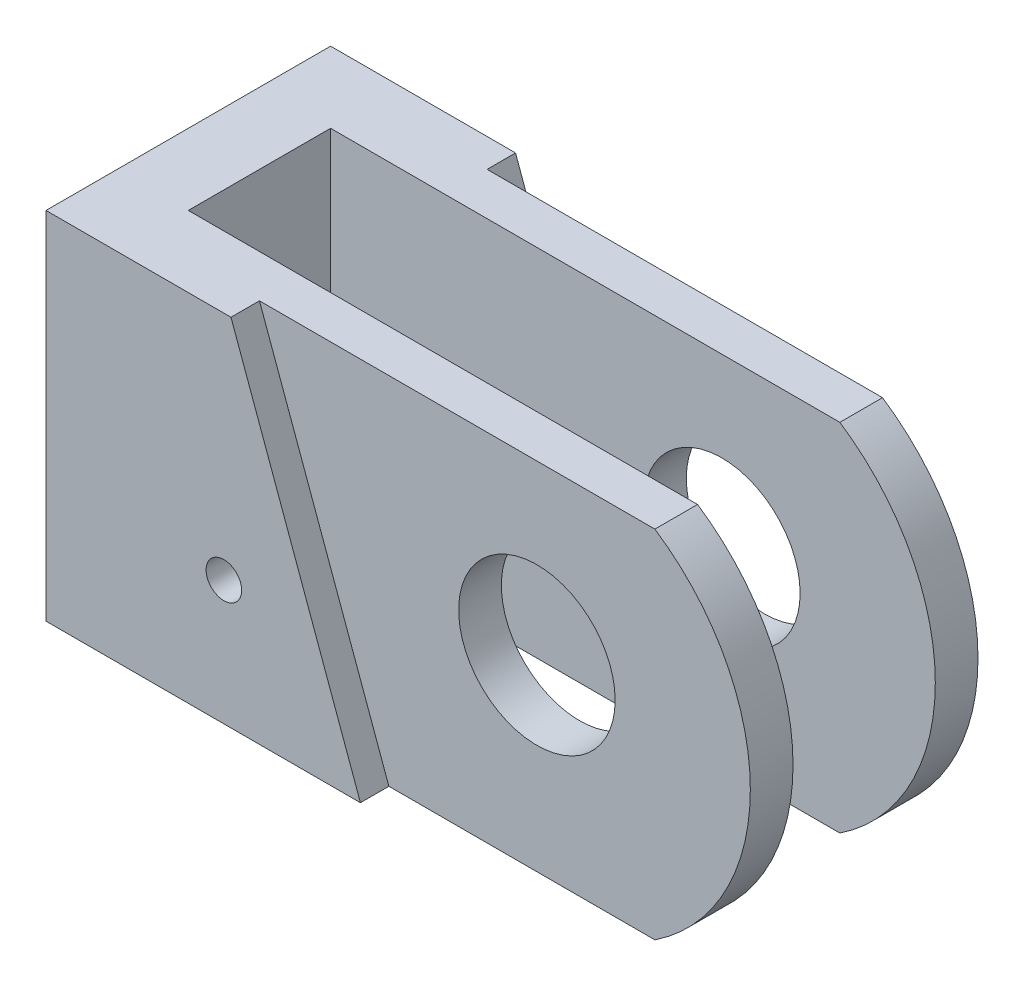
ISO-10303-21;
HEADER;
FILE_DESCRIPTION(('STEP AP214'),'2;1');
FILE_NAME('part.step','',(''),(''),'','','');
FILE_SCHEMA(('AUTOMOTIVE_DESIGN { 1 0 10303 214 1 1 1 1 }'));
ENDSEC;
DATA;
#1=APPLICATION_CONTEXT('core data for automotive mechanical design processes');
#2=APPLICATION_PROTOCOL_DEFINITION('international standard','automotive_design',2000,#1);
#3=PRODUCT_CONTEXT('',#1,'mechanical');
#4=PRODUCT('Part','Part','',(#3));
#5=PRODUCT_RELATED_PRODUCT_CATEGORY('part','',(#4));
#6=PRODUCT_DEFINITION_FORMATION('','',#4);
#7=PRODUCT_DEFINITION_CONTEXT('part definition',#1,'design');
#8=PRODUCT_DEFINITION('design','',#6,#7);
#9=PRODUCT_DEFINITION_SHAPE('','',#8);
#10=(LENGTH_UNIT() NAMED_UNIT(*) SI_UNIT(.MILLI.,.METRE.));
#11=(NAMED_UNIT(*) PLANE_ANGLE_UNIT() SI_UNIT($,.RADIAN.));
#12=(NAMED_UNIT(*) SI_UNIT($,.STERADIAN.) SOLID_ANGLE_UNIT());
#13=UNCERTAINTY_MEASURE_WITH_UNIT(LENGTH_MEASURE(1.E-05),#10,'distance_accuracy_value','');
#14=(GEOMETRIC_REPRESENTATION_CONTEXT(3) GLOBAL_UNCERTAINTY_ASSIGNED_CONTEXT((#13)) GLOBAL_UNIT_ASSIGNED_CONTEXT((#10,
#11,#12)) REPRESENTATION_CONTEXT('',''));
#15=CARTESIAN_POINT('',(0.,0.,0.));
#16=DIRECTION('',(0.,0.,1.));
#17=DIRECTION('',(1.,0.,0.));
#18=AXIS2_PLACEMENT_3D('',#15,#16,#17);
#19=CARTESIAN_POINT('',(10.,0.,0.));
#20=DIRECTION('',(1.,0.,0.));
#21=DIRECTION('',(0.,1.,0.));
#22=AXIS2_PLACEMENT_3D('',#19,#20,#21);
#23=PLANE('',#22);
#24=CARTESIAN_POINT('',(10.,-25.,20.));
#25=DIRECTION('',(1.,0.,0.));
#26=DIRECTION('',(0.,1.,0.));
#27=AXIS2_PLACEMENT_3D('',#24,#25,#26);
#28=CIRCLE('',#27,10.);
#29=CARTESIAN_POINT('',(10.,-25.,30.));
#30=VERTEX_POINT('',#29);
#31=CARTESIAN_POINT('',(10.,-25.,10.));
#32=VERTEX_POINT('',#31);
#33=EDGE_CURVE('E64',#30,#32,#28,.T.);
#34=ORIENTED_EDGE('',*,*,#33,.F.);
#35=DIRECTION('',(0.,-1.,0.));
#36=VECTOR('',#35,1.);
#37=CARTESIAN_POINT('',(10.,-50.,30.));
#38=LINE('',#37,#36);
#39=CARTESIAN_POINT('',(10.,-50.,30.));
#40=VERTEX_POINT('',#39);
#41=EDGE_CURVE('E151',#30,#40,#38,.T.);
#42=ORIENTED_EDGE('',*,*,#41,.T.);
#43=DIRECTION('',(0.,0.,1.));
#44=VECTOR('',#43,1.);
#45=CARTESIAN_POINT('',(10.,-50.,40.));
#46=LINE('',#45,#44);
#47=CARTESIAN_POINT('',(10.,-50.,10.));
#48=VERTEX_POINT('',#47);
#49=EDGE_CURVE('E188',#48,#40,#46,.T.);
#50=ORIENTED_EDGE('',*,*,#49,.F.);
#51=DIRECTION('',(0.,-1.,0.));
#52=VECTOR('',#51,1.);
#53=CARTESIAN_POINT('',(10.,-50.,10.));
#54=LINE('',#53,#52);
#55=EDGE_CURVE('E153',#32,#48,#54,.T.);
#56=ORIENTED_EDGE('',*,*,#55,.F.);
#57=EDGE_LOOP('',(#34,#42,#50,#56));
#58=FACE_BOUND('',#57,.T.);
#59=ADVANCED_FACE('F44',(#58),#23,.T.);
#60=CARTESIAN_POINT('',(65.,-25.,10.));
#61=DIRECTION('',(0.,0.,-1.));
#62=DIRECTION('',(-1.,0.,0.));
#63=AXIS2_PLACEMENT_3D('',#60,#61,#62);
#64=CYLINDRICAL_SURFACE('',#63,30.);
#65=CARTESIAN_POINT('',(65.,-25.,4.));
#66=DIRECTION('',(0.,0.,-1.));
#67=DIRECTION('',(-1.,0.,0.));
#68=AXIS2_PLACEMENT_3D('',#65,#66,#67);
#69=CIRCLE('',#68,30.);
#70=CARTESIAN_POINT('',(81.583123951777,0.,4.));
#71=VERTEX_POINT('',#70);
#72=CARTESIAN_POINT('',(81.583123951777,-50.,4.));
#73=VERTEX_POINT('',#72);
#74=EDGE_CURVE('E252',#71,#73,#69,.T.);
#75=ORIENTED_EDGE('',*,*,#74,.F.);
#76=DIRECTION('',(0.,0.,-1.));
#77=VECTOR('',#76,1.);
#78=CARTESIAN_POINT('',(81.583123951777,0.,10.));
#79=LINE('',#78,#77);
#80=CARTESIAN_POINT('',(81.583123951777,0.,10.));
#81=VERTEX_POINT('',#80);
#82=EDGE_CURVE('E209',#81,#71,#79,.T.);
#83=ORIENTED_EDGE('',*,*,#82,.F.);
#84=CARTESIAN_POINT('',(65.,-25.,10.));
#85=DIRECTION('',(0.,0.,1.));
#86=DIRECTION('',(1.,0.,0.));
#87=AXIS2_PLACEMENT_3D('',#84,#85,#86);
#88=CIRCLE('',#87,30.);
#89=CARTESIAN_POINT('',(81.583123951777,-50.,10.));
#90=VERTEX_POINT('',#89);
#91=EDGE_CURVE('E207',#90,#81,#88,.T.);
#92=ORIENTED_EDGE('',*,*,#91,.F.);
#93=DIRECTION('',(0.,0.,-1.));
#94=VECTOR('',#93,1.);
#95=CARTESIAN_POINT('',(81.583123951777,-50.,10.));
#96=LINE('',#95,#94);
#97=EDGE_CURVE('E218',#90,#73,#96,.T.);
#98=ORIENTED_EDGE('',*,*,#97,.T.);
#99=EDGE_LOOP('',(#75,#83,#92,#98));
#100=FACE_BOUND('',#99,.T.);
#101=ADVANCED_FACE('F297',(#100),#64,.T.);
#102=CARTESIAN_POINT('',(65.,-25.,30.));
#103=DIRECTION('',(0.,0.,1.));
#104=DIRECTION('',(1.,0.,0.));
#105=AXIS2_PLACEMENT_3D('',#102,#103,#104);
#106=CYLINDRICAL_SURFACE('',#105,30.);
#107=DIRECTION('',(0.,0.,1.));
#108=VECTOR('',#107,1.);
#109=CARTESIAN_POINT('',(81.583123951777,0.,30.));
#110=LINE('',#109,#108);
#111=CARTESIAN_POINT('',(81.583123951777,0.,30.));
#112=VERTEX_POINT('',#111);
#113=CARTESIAN_POINT('',(81.583123951777,0.,36.));
#114=VERTEX_POINT('',#113);
#115=EDGE_CURVE('E185',#112,#114,#110,.T.);
#116=ORIENTED_EDGE('',*,*,#115,.T.);
#117=CARTESIAN_POINT('',(65.,-25.,36.));
#118=DIRECTION('',(0.,0.,1.));
#119=DIRECTION('',(1.,0.,0.));
#120=AXIS2_PLACEMENT_3D('',#117,#118,#119);
#121=CIRCLE('',#120,30.);
#122=CARTESIAN_POINT('',(81.583123951777,-50.,36.));
#123=VERTEX_POINT('',#122);
#124=EDGE_CURVE('E269',#123,#114,#121,.T.);
#125=ORIENTED_EDGE('',*,*,#124,.F.);
#126=DIRECTION('',(0.,0.,1.));
#127=VECTOR('',#126,1.);
#128=CARTESIAN_POINT('',(81.583123951777,-50.,30.));
#129=LINE('',#128,#127);
#130=CARTESIAN_POINT('',(81.583123951777,-50.,30.));
#131=VERTEX_POINT('',#130);
#132=EDGE_CURVE('E181',#131,#123,#129,.T.);
#133=ORIENTED_EDGE('',*,*,#132,.F.);
#134=CARTESIAN_POINT('',(65.,-25.,30.));
#135=DIRECTION('',(0.,0.,1.));
#136=DIRECTION('',(1.,0.,0.));
#137=AXIS2_PLACEMENT_3D('',#134,#135,#136);
#138=CIRCLE('',#137,30.);
#139=EDGE_CURVE('E171',#131,#112,#138,.T.);
#140=ORIENTED_EDGE('',*,*,#139,.T.);
#141=EDGE_LOOP('',(#116,#125,#133,#140));
#142=FACE_BOUND('',#141,.T.);
#143=ADVANCED_FACE('F307',(#142),#106,.T.);
#144=EDGE_CURVE('E136',#32,#30,#28,.T.);
#145=ORIENTED_EDGE('',*,*,#144,.F.);
#146=CARTESIAN_POINT('',(10.,0.,10.));
#147=VERTEX_POINT('',#146);
#148=EDGE_CURVE('E189',#147,#32,#54,.T.);
#149=ORIENTED_EDGE('',*,*,#148,.F.);
#150=DIRECTION('',(0.,0.,-1.));
#151=VECTOR('',#150,1.);
#152=CARTESIAN_POINT('',(10.,0.,10.));
#153=LINE('',#152,#151);
#154=CARTESIAN_POINT('',(10.,0.,30.));
#155=VERTEX_POINT('',#154);
#156=EDGE_CURVE('E167',#155,#147,#153,.T.);
#157=ORIENTED_EDGE('',*,*,#156,.F.);
#158=EDGE_CURVE('E158',#155,#30,#38,.T.);
#159=ORIENTED_EDGE('',*,*,#158,.T.);
#160=EDGE_LOOP('',(#145,#149,#157,#159));
#161=FACE_BOUND('',#160,.T.);
#162=ADVANCED_FACE('F169',(#161),#23,.T.);
#163=CARTESIAN_POINT('',(65.,-25.,10.));
#164=DIRECTION('',(0.,0.,1.));
#165=DIRECTION('',(1.,0.,0.));
#166=AXIS2_PLACEMENT_3D('',#163,#164,#165);
#167=PLANE('',#166);
#168=CARTESIAN_POINT('',(25.,-32.5,10.));
#169=DIRECTION('',(0.,0.,1.));
#170=DIRECTION('',(1.,0.,0.));
#171=AXIS2_PLACEMENT_3D('',#168,#169,#170);
#172=CIRCLE('',#171,2.5);
#173=CARTESIAN_POINT('',(27.5,-32.5,10.));
#174=VERTEX_POINT('',#173);
#175=EDGE_CURVE('E354',#174,#174,#172,.T.);
#176=ORIENTED_EDGE('',*,*,#175,.F.);
#177=EDGE_LOOP('',(#176));
#178=FACE_BOUND('',#177,.T.);
#179=ORIENTED_EDGE('',*,*,#148,.T.);
#180=ORIENTED_EDGE('',*,*,#55,.T.);
#181=DIRECTION('',(1.,0.,0.));
#182=VECTOR('',#181,1.);
#183=CARTESIAN_POINT('',(0.,-50.,10.));
#184=LINE('',#183,#182);
#185=EDGE_CURVE('E205',#48,#90,#184,.T.);
#186=ORIENTED_EDGE('',*,*,#185,.T.);
#187=ORIENTED_EDGE('',*,*,#91,.T.);
#188=DIRECTION('',(-1.,0.,0.));
#189=VECTOR('',#188,1.);
#190=CARTESIAN_POINT('',(0.,0.,10.));
#191=LINE('',#190,#189);
#192=EDGE_CURVE('E199',#81,#147,#191,.T.);
#193=ORIENTED_EDGE('',*,*,#192,.T.);
#194=EDGE_LOOP('',(#179,#180,#186,#187,#193));
#195=FACE_BOUND('',#194,.T.);
#196=CARTESIAN_POINT('',(65.,-23.6191908710067,10.));
#197=DIRECTION('',(0.,0.,1.));
#198=DIRECTION('',(1.,0.,0.));
#199=AXIS2_PLACEMENT_3D('',#196,#197,#198);
#200=CIRCLE('',#199,11.);
#201=CARTESIAN_POINT('',(76.,-23.6191908710067,10.));
#202=VERTEX_POINT('',#201);
#203=EDGE_CURVE('E230',#202,#202,#200,.T.);
#204=ORIENTED_EDGE('',*,*,#203,.F.);
#205=EDGE_LOOP('',(#204));
#206=FACE_BOUND('',#205,.T.);
#207=ADVANCED_FACE('F304',(#178,#195,#206),#167,.T.);
#208=CARTESIAN_POINT('',(0.,0.,10.));
#209=DIRECTION('',(1.,0.,0.));
#210=DIRECTION('',(0.,1.,0.));
#211=AXIS2_PLACEMENT_3D('',#208,#209,#210);
#212=PLANE('',#211);
#213=CARTESIAN_POINT('',(0.,-25.,20.));
#214=DIRECTION('',(-1.,0.,0.));
#215=DIRECTION('',(0.,-1.,0.));
#216=AXIS2_PLACEMENT_3D('',#213,#214,#215);
#217=CIRCLE('',#216,15.);
#218=CARTESIAN_POINT('',(0.,-40.,20.));
#219=VERTEX_POINT('',#218);
#220=EDGE_CURVE('E154',#219,#219,#217,.T.);
#221=ORIENTED_EDGE('',*,*,#220,.F.);
#222=EDGE_LOOP('',(#221));
#223=FACE_BOUND('',#222,.T.);
#224=DIRECTION('',(0.,-1.,0.));
#225=VECTOR('',#224,1.);
#226=CARTESIAN_POINT('',(0.,0.,0.));
#227=LINE('',#226,#225);
#228=CARTESIAN_POINT('',(0.,0.,0.));
#229=VERTEX_POINT('',#228);
#230=CARTESIAN_POINT('',(0.,-50.,0.));
#231=VERTEX_POINT('',#230);
#232=EDGE_CURVE('E198',#229,#231,#227,.T.);
#233=ORIENTED_EDGE('',*,*,#232,.T.);
#234=DIRECTION('',(0.,0.,-1.));
#235=VECTOR('',#234,1.);
#236=CARTESIAN_POINT('',(0.,-50.,10.));
#237=LINE('',#236,#235);
#238=CARTESIAN_POINT('',(0.,-50.,40.));
#239=VERTEX_POINT('',#238);
#240=EDGE_CURVE('E53',#239,#231,#237,.T.);
#241=ORIENTED_EDGE('',*,*,#240,.F.);
#242=DIRECTION('',(0.,1.,0.));
#243=VECTOR('',#242,1.);
#244=CARTESIAN_POINT('',(0.,0.,40.));
#245=LINE('',#244,#243);
#246=CARTESIAN_POINT('',(0.,0.,40.));
#247=VERTEX_POINT('',#246);
#248=EDGE_CURVE('E184',#239,#247,#245,.T.);
#249=ORIENTED_EDGE('',*,*,#248,.T.);
#250=DIRECTION('',(0.,0.,-1.));
#251=VECTOR('',#250,1.);
#252=CARTESIAN_POINT('',(0.,0.,10.));
#253=LINE('',#252,#251);
#254=EDGE_CURVE('E11',#247,#229,#253,.T.);
#255=ORIENTED_EDGE('',*,*,#254,.T.);
#256=EDGE_LOOP('',(#233,#241,#249,#255));
#257=FACE_BOUND('',#256,.T.);
#258=ADVANCED_FACE('F50',(#223,#257),#212,.F.);
#259=CARTESIAN_POINT('',(77.2892753227361,-50.,10.));
#260=DIRECTION('',(0.,1.,0.));
#261=DIRECTION('',(-1.,0.,0.));
#262=AXIS2_PLACEMENT_3D('',#259,#260,#261);
#263=PLANE('',#262);
#264=DIRECTION('',(1.,0.,0.));
#265=VECTOR('',#264,1.);
#266=CARTESIAN_POINT('',(77.2892753227361,-50.,0.));
#267=LINE('',#266,#265);
#268=CARTESIAN_POINT('',(44.2,-50.0000000000001,0.));
#269=VERTEX_POINT('',#268);
#270=EDGE_CURVE('E211',#231,#269,#267,.T.);
#271=ORIENTED_EDGE('',*,*,#270,.T.);
#272=DIRECTION('',(0.,0.,-1.));
#273=VECTOR('',#272,1.);
#274=CARTESIAN_POINT('',(44.2,-50.,4.));
#275=LINE('',#274,#273);
#276=CARTESIAN_POINT('',(44.2,-50.,4.));
#277=VERTEX_POINT('',#276);
#278=EDGE_CURVE('E67',#277,#269,#275,.T.);
#279=ORIENTED_EDGE('',*,*,#278,.F.);
#280=DIRECTION('',(-1.,0.,0.));
#281=VECTOR('',#280,1.);
#282=CARTESIAN_POINT('',(81.583123951777,-50.,4.));
#283=LINE('',#282,#281);
#284=EDGE_CURVE('E243',#73,#277,#283,.T.);
#285=ORIENTED_EDGE('',*,*,#284,.F.);
#286=ORIENTED_EDGE('',*,*,#97,.F.);
#287=ORIENTED_EDGE('',*,*,#185,.F.);
#288=ORIENTED_EDGE('',*,*,#49,.T.);
#289=DIRECTION('',(1.,0.,0.));
#290=VECTOR('',#289,1.);
#291=CARTESIAN_POINT('',(81.583123951777,-50.,30.));
#292=LINE('',#291,#290);
#293=EDGE_CURVE('E165',#40,#131,#292,.T.);
#294=ORIENTED_EDGE('',*,*,#293,.T.);
#295=ORIENTED_EDGE('',*,*,#132,.T.);
#296=DIRECTION('',(1.,0.,0.));
#297=VECTOR('',#296,1.);
#298=CARTESIAN_POINT('',(0.,-50.,36.));
#299=LINE('',#298,#297);
#300=CARTESIAN_POINT('',(44.196790464873,-50.,36.));
#301=VERTEX_POINT('',#300);
#302=EDGE_CURVE('E264',#301,#123,#299,.T.);
#303=ORIENTED_EDGE('',*,*,#302,.F.);
#304=DIRECTION('',(0.,0.,1.));
#305=VECTOR('',#304,1.);
#306=CARTESIAN_POINT('',(44.196790464873,-50.,36.));
#307=LINE('',#306,#305);
#308=CARTESIAN_POINT('',(44.196790464873,-50.,40.));
#309=VERTEX_POINT('',#308);
#310=EDGE_CURVE('E168',#301,#309,#307,.T.);
#311=ORIENTED_EDGE('',*,*,#310,.T.);
#312=DIRECTION('',(-1.,0.,0.));
#313=VECTOR('',#312,1.);
#314=CARTESIAN_POINT('',(10.,-50.,40.));
#315=LINE('',#314,#313);
#316=EDGE_CURVE('E195',#309,#239,#315,.T.);
#317=ORIENTED_EDGE('',*,*,#316,.T.);
#318=ORIENTED_EDGE('',*,*,#240,.T.);
#319=EDGE_LOOP('',(#271,#279,#285,#286,#287,#288,#294,#295,#303,#311,#317,#318));
#320=FACE_BOUND('',#319,.T.);
#321=ADVANCED_FACE('F288',(#320),#263,.F.);
#322=CARTESIAN_POINT('',(61.578947368421,0.,10.));
#323=DIRECTION('',(0.,-1.,0.));
#324=DIRECTION('',(0.,0.,-1.));
#325=AXIS2_PLACEMENT_3D('',#322,#323,#324);
#326=PLANE('',#325);
#327=DIRECTION('',(1.,0.,0.));
#328=VECTOR('',#327,1.);
#329=CARTESIAN_POINT('',(26.,0.,4.));
#330=LINE('',#329,#328);
#331=CARTESIAN_POINT('',(26.,0.,4.));
#332=VERTEX_POINT('',#331);
#333=EDGE_CURVE('E248',#332,#71,#330,.T.);
#334=ORIENTED_EDGE('',*,*,#333,.F.);
#335=DIRECTION('',(0.,0.,-1.));
#336=VECTOR('',#335,1.);
#337=CARTESIAN_POINT('',(26.,0.,4.));
#338=LINE('',#337,#336);
#339=CARTESIAN_POINT('',(26.,0.,0.));
#340=VERTEX_POINT('',#339);
#341=EDGE_CURVE('E251',#332,#340,#338,.T.);
#342=ORIENTED_EDGE('',*,*,#341,.T.);
#343=DIRECTION('',(-1.,0.,0.));
#344=VECTOR('',#343,1.);
#345=CARTESIAN_POINT('',(61.578947368421,0.,0.));
#346=LINE('',#345,#344);
#347=EDGE_CURVE('E201',#340,#229,#346,.T.);
#348=ORIENTED_EDGE('',*,*,#347,.T.);
#349=ORIENTED_EDGE('',*,*,#254,.F.);
#350=DIRECTION('',(-1.,0.,0.));
#351=VECTOR('',#350,1.);
#352=CARTESIAN_POINT('',(10.,0.,40.));
#353=LINE('',#352,#351);
#354=CARTESIAN_POINT('',(26.,0.,40.));
#355=VERTEX_POINT('',#354);
#356=EDGE_CURVE('E196',#355,#247,#353,.T.);
#357=ORIENTED_EDGE('',*,*,#356,.F.);
#358=DIRECTION('',(0.,0.,1.));
#359=VECTOR('',#358,1.);
#360=CARTESIAN_POINT('',(26.,0.,36.));
#361=LINE('',#360,#359);
#362=CARTESIAN_POINT('',(26.,0.,36.));
#363=VERTEX_POINT('',#362);
#364=EDGE_CURVE('E172',#363,#355,#361,.T.);
#365=ORIENTED_EDGE('',*,*,#364,.F.);
#366=DIRECTION('',(-1.,0.,0.));
#367=VECTOR('',#366,1.);
#368=CARTESIAN_POINT('',(0.,0.,36.));
#369=LINE('',#368,#367);
#370=EDGE_CURVE('E258',#114,#363,#369,.T.);
#371=ORIENTED_EDGE('',*,*,#370,.F.);
#372=ORIENTED_EDGE('',*,*,#115,.F.);
#373=DIRECTION('',(-1.,0.,0.));
#374=VECTOR('',#373,1.);
#375=CARTESIAN_POINT('',(10.,0.,30.));
#376=LINE('',#375,#374);
#377=EDGE_CURVE('E177',#112,#155,#376,.T.);
#378=ORIENTED_EDGE('',*,*,#377,.T.);
#379=ORIENTED_EDGE('',*,*,#156,.T.);
#380=ORIENTED_EDGE('',*,*,#192,.F.);
#381=ORIENTED_EDGE('',*,*,#82,.T.);
#382=EDGE_LOOP('',(#334,#342,#348,#349,#357,#365,#371,#372,#378,#379,#380,#381));
#383=FACE_BOUND('',#382,.T.);
#384=ADVANCED_FACE('F284',(#383),#326,.F.);
#385=CARTESIAN_POINT('',(65.,-25.,0.));
#386=DIRECTION('',(0.,0.,1.));
#387=DIRECTION('',(1.,0.,0.));
#388=AXIS2_PLACEMENT_3D('',#385,#386,#387);
#389=PLANE('',#388);
#390=CARTESIAN_POINT('',(25.,-32.5,0.));
#391=DIRECTION('',(0.,0.,1.));
#392=DIRECTION('',(1.,0.,0.));
#393=AXIS2_PLACEMENT_3D('',#390,#391,#392);
#394=CIRCLE('',#393,2.5);
#395=CARTESIAN_POINT('',(27.5,-32.5,0.));
#396=VERTEX_POINT('',#395);
#397=EDGE_CURVE('E355',#396,#396,#394,.T.);
#398=ORIENTED_EDGE('',*,*,#397,.T.);
#399=EDGE_LOOP('',(#398));
#400=FACE_BOUND('',#399,.T.);
#401=ORIENTED_EDGE('',*,*,#347,.F.);
#402=DIRECTION('',(-0.34204484166827,0.939683630956785,0.));
#403=VECTOR('',#402,1.);
#404=CARTESIAN_POINT('',(26.,0.,0.));
#405=LINE('',#404,#403);
#406=EDGE_CURVE('E245',#269,#340,#405,.T.);
#407=ORIENTED_EDGE('',*,*,#406,.F.);
#408=ORIENTED_EDGE('',*,*,#270,.F.);
#409=ORIENTED_EDGE('',*,*,#232,.F.);
#410=EDGE_LOOP('',(#401,#407,#408,#409));
#411=FACE_BOUND('',#410,.T.);
#412=ADVANCED_FACE('F291',(#400,#411),#389,.F.);
#413=CARTESIAN_POINT('',(10.,0.,40.));
#414=DIRECTION('',(0.,0.,1.));
#415=DIRECTION('',(1.,0.,0.));
#416=AXIS2_PLACEMENT_3D('',#413,#414,#415);
#417=PLANE('',#416);
#418=CARTESIAN_POINT('',(25.,-32.5,40.));
#419=DIRECTION('',(0.,0.,1.));
#420=DIRECTION('',(1.,0.,0.));
#421=AXIS2_PLACEMENT_3D('',#418,#419,#420);
#422=CIRCLE('',#421,2.5);
#423=CARTESIAN_POINT('',(27.5,-32.5,40.));
#424=VERTEX_POINT('',#423);
#425=EDGE_CURVE('E357',#424,#424,#422,.T.);
#426=ORIENTED_EDGE('',*,*,#425,.F.);
#427=EDGE_LOOP('',(#426));
#428=FACE_BOUND('',#427,.T.);
#429=DIRECTION('',(0.341991578063699,-0.939703017199318,0.));
#430=VECTOR('',#429,1.);
#431=CARTESIAN_POINT('',(22.959085773871,8.35563346184355,40.));
#432=LINE('',#431,#430);
#433=EDGE_CURVE('E256',#355,#309,#432,.T.);
#434=ORIENTED_EDGE('',*,*,#433,.F.);
#435=ORIENTED_EDGE('',*,*,#356,.T.);
#436=ORIENTED_EDGE('',*,*,#248,.F.);
#437=ORIENTED_EDGE('',*,*,#316,.F.);
#438=EDGE_LOOP('',(#434,#435,#436,#437));
#439=FACE_BOUND('',#438,.T.);
#440=ADVANCED_FACE('F281',(#428,#439),#417,.T.);
#441=CARTESIAN_POINT('',(65.,-25.,30.));
#442=DIRECTION('',(0.,0.,1.));
#443=DIRECTION('',(1.,0.,0.));
#444=AXIS2_PLACEMENT_3D('',#441,#442,#443);
#445=PLANE('',#444);
#446=CARTESIAN_POINT('',(25.,-32.5,30.));
#447=DIRECTION('',(0.,0.,1.));
#448=DIRECTION('',(1.,0.,0.));
#449=AXIS2_PLACEMENT_3D('',#446,#447,#448);
#450=CIRCLE('',#449,2.5);
#451=CARTESIAN_POINT('',(27.5,-32.5,30.));
#452=VERTEX_POINT('',#451);
#453=EDGE_CURVE('E47',#452,#452,#450,.T.);
#454=ORIENTED_EDGE('',*,*,#453,.T.);
#455=EDGE_LOOP('',(#454));
#456=FACE_BOUND('',#455,.T.);
#457=ORIENTED_EDGE('',*,*,#41,.F.);
#458=ORIENTED_EDGE('',*,*,#158,.F.);
#459=ORIENTED_EDGE('',*,*,#377,.F.);
#460=ORIENTED_EDGE('',*,*,#139,.F.);
#461=ORIENTED_EDGE('',*,*,#293,.F.);
#462=EDGE_LOOP('',(#457,#458,#459,#460,#461));
#463=FACE_BOUND('',#462,.T.);
#464=CARTESIAN_POINT('',(65.,-23.6191908710067,30.));
#465=DIRECTION('',(0.,0.,1.));
#466=DIRECTION('',(1.,0.,0.));
#467=AXIS2_PLACEMENT_3D('',#464,#465,#466);
#468=CIRCLE('',#467,11.);
#469=CARTESIAN_POINT('',(76.,-23.6191908710067,30.));
#470=VERTEX_POINT('',#469);
#471=EDGE_CURVE('E221',#470,#470,#468,.T.);
#472=ORIENTED_EDGE('',*,*,#471,.T.);
#473=EDGE_LOOP('',(#472));
#474=FACE_BOUND('',#473,.T.);
#475=ADVANCED_FACE('F159',(#456,#463,#474),#445,.F.);
#476=CARTESIAN_POINT('',(22.959085773871,8.35563346184355,36.));
#477=DIRECTION('',(-0.939703017199318,-0.341991578063699,0.));
#478=DIRECTION('',(0.341991578063699,-0.939703017199318,0.));
#479=AXIS2_PLACEMENT_3D('',#476,#477,#478);
#480=PLANE('',#479);
#481=ORIENTED_EDGE('',*,*,#433,.T.);
#482=ORIENTED_EDGE('',*,*,#310,.F.);
#483=DIRECTION('',(0.341991578063699,-0.939703017199318,0.));
#484=VECTOR('',#483,1.);
#485=CARTESIAN_POINT('',(22.959085773871,8.35563346184355,36.));
#486=LINE('',#485,#484);
#487=EDGE_CURVE('E265',#363,#301,#486,.T.);
#488=ORIENTED_EDGE('',*,*,#487,.F.);
#489=ORIENTED_EDGE('',*,*,#364,.T.);
#490=EDGE_LOOP('',(#481,#482,#488,#489));
#491=FACE_BOUND('',#490,.T.);
#492=ADVANCED_FACE('F279',(#491),#480,.F.);
#493=CARTESIAN_POINT('',(0.,0.,36.));
#494=DIRECTION('',(0.,0.,1.));
#495=DIRECTION('',(1.,0.,0.));
#496=AXIS2_PLACEMENT_3D('',#493,#494,#495);
#497=PLANE('',#496);
#498=CARTESIAN_POINT('',(65.,-23.6191908710067,36.));
#499=DIRECTION('',(0.,0.,1.));
#500=DIRECTION('',(1.,0.,0.));
#501=AXIS2_PLACEMENT_3D('',#498,#499,#500);
#502=CIRCLE('',#501,11.);
#503=CARTESIAN_POINT('',(76.,-23.6191908710067,36.));
#504=VERTEX_POINT('',#503);
#505=EDGE_CURVE('E223',#504,#504,#502,.T.);
#506=ORIENTED_EDGE('',*,*,#505,.F.);
#507=EDGE_LOOP('',(#506));
#508=FACE_BOUND('',#507,.T.);
#509=ORIENTED_EDGE('',*,*,#370,.T.);
#510=ORIENTED_EDGE('',*,*,#487,.T.);
#511=ORIENTED_EDGE('',*,*,#302,.T.);
#512=ORIENTED_EDGE('',*,*,#124,.T.);
#513=EDGE_LOOP('',(#509,#510,#511,#512));
#514=FACE_BOUND('',#513,.T.);
#515=ADVANCED_FACE('F311',(#508,#514),#497,.T.);
#516=CARTESIAN_POINT('',(26.,0.,4.));
#517=DIRECTION('',(-0.939683630956786,-0.34204484166827,0.));
#518=DIRECTION('',(0.34204484166827,-0.939683630956785,0.));
#519=AXIS2_PLACEMENT_3D('',#516,#517,#518);
#520=PLANE('',#519);
#521=ORIENTED_EDGE('',*,*,#406,.T.);
#522=ORIENTED_EDGE('',*,*,#341,.F.);
#523=DIRECTION('',(-0.34204484166827,0.939683630956785,0.));
#524=VECTOR('',#523,1.);
#525=CARTESIAN_POINT('',(26.,0.,4.));
#526=LINE('',#525,#524);
#527=EDGE_CURVE('E246',#277,#332,#526,.T.);
#528=ORIENTED_EDGE('',*,*,#527,.F.);
#529=ORIENTED_EDGE('',*,*,#278,.T.);
#530=EDGE_LOOP('',(#521,#522,#528,#529));
#531=FACE_BOUND('',#530,.T.);
#532=ADVANCED_FACE('F295',(#531),#520,.F.);
#533=CARTESIAN_POINT('',(65.,-25.,4.));
#534=DIRECTION('',(0.,0.,-1.));
#535=DIRECTION('',(-1.,0.,0.));
#536=AXIS2_PLACEMENT_3D('',#533,#534,#535);
#537=PLANE('',#536);
#538=CARTESIAN_POINT('',(65.,-23.6191908710067,4.));
#539=DIRECTION('',(0.,0.,-1.));
#540=DIRECTION('',(-1.,0.,0.));
#541=AXIS2_PLACEMENT_3D('',#538,#539,#540);
#542=CIRCLE('',#541,11.);
#543=CARTESIAN_POINT('',(54.,-23.6191908710067,4.));
#544=VERTEX_POINT('',#543);
#545=EDGE_CURVE('E224',#544,#544,#542,.T.);
#546=ORIENTED_EDGE('',*,*,#545,.F.);
#547=EDGE_LOOP('',(#546));
#548=FACE_BOUND('',#547,.T.);
#549=ORIENTED_EDGE('',*,*,#284,.T.);
#550=ORIENTED_EDGE('',*,*,#527,.T.);
#551=ORIENTED_EDGE('',*,*,#333,.T.);
#552=ORIENTED_EDGE('',*,*,#74,.T.);
#553=EDGE_LOOP('',(#549,#550,#551,#552));
#554=FACE_BOUND('',#553,.T.);
#555=ADVANCED_FACE('F296',(#548,#554),#537,.T.);
#556=CARTESIAN_POINT('',(65.,-23.6191908710067,-4.));
#557=DIRECTION('',(0.,0.,1.));
#558=DIRECTION('',(1.,0.,0.));
#559=AXIS2_PLACEMENT_3D('',#556,#557,#558);
#560=CYLINDRICAL_SURFACE('',#559,11.);
#561=ORIENTED_EDGE('',*,*,#203,.T.);
#562=EDGE_LOOP('',(#561));
#563=FACE_BOUND('',#562,.T.);
#564=ORIENTED_EDGE('',*,*,#545,.T.);
#565=EDGE_LOOP('',(#564));
#566=FACE_BOUND('',#565,.T.);
#567=ADVANCED_FACE('F460',(#563,#566),#560,.F.);
#568=ORIENTED_EDGE('',*,*,#505,.T.);
#569=EDGE_LOOP('',(#568));
#570=FACE_BOUND('',#569,.T.);
#571=ORIENTED_EDGE('',*,*,#471,.F.);
#572=EDGE_LOOP('',(#571));
#573=FACE_BOUND('',#572,.T.);
#574=ADVANCED_FACE('F376',(#570,#573),#560,.F.);
#575=CARTESIAN_POINT('',(2.,-25.,20.));
#576=DIRECTION('',(-1.,0.,0.));
#577=DIRECTION('',(0.,-1.,0.));
#578=AXIS2_PLACEMENT_3D('',#575,#576,#577);
#579=CYLINDRICAL_SURFACE('',#578,15.);
#580=CARTESIAN_POINT('',(2.,-25.,20.));
#581=DIRECTION('',(-1.,0.,0.));
#582=DIRECTION('',(0.,-1.,0.));
#583=AXIS2_PLACEMENT_3D('',#580,#581,#582);
#584=CIRCLE('',#583,15.);
#585=CARTESIAN_POINT('',(2.,-40.,20.));
#586=VERTEX_POINT('',#585);
#587=EDGE_CURVE('E235',#586,#586,#584,.T.);
#588=ORIENTED_EDGE('',*,*,#587,.F.);
#589=EDGE_LOOP('',(#588));
#590=FACE_BOUND('',#589,.T.);
#591=ORIENTED_EDGE('',*,*,#220,.T.);
#592=EDGE_LOOP('',(#591));
#593=FACE_BOUND('',#592,.T.);
#594=ADVANCED_FACE('F369',(#590,#593),#579,.F.);
#595=CARTESIAN_POINT('',(2.,-25.,20.));
#596=DIRECTION('',(-1.,0.,0.));
#597=DIRECTION('',(0.,-1.,0.));
#598=AXIS2_PLACEMENT_3D('',#595,#596,#597);
#599=PLANE('',#598);
#600=CARTESIAN_POINT('',(2.,-25.,20.));
#601=DIRECTION('',(-1.,0.,0.));
#602=DIRECTION('',(0.,-1.,0.));
#603=AXIS2_PLACEMENT_3D('',#600,#601,#602);
#604=CIRCLE('',#603,10.);
#605=CARTESIAN_POINT('',(2.,-35.,20.));
#606=VERTEX_POINT('',#605);
#607=EDGE_CURVE('E149',#606,#606,#604,.T.);
#608=ORIENTED_EDGE('',*,*,#607,.F.);
#609=EDGE_LOOP('',(#608));
#610=FACE_BOUND('',#609,.T.);
#611=ORIENTED_EDGE('',*,*,#587,.T.);
#612=EDGE_LOOP('',(#611));
#613=FACE_BOUND('',#612,.T.);
#614=ADVANCED_FACE('F370',(#610,#613),#599,.T.);
#615=CARTESIAN_POINT('',(17.,-25.,20.));
#616=DIRECTION('',(-1.,0.,0.));
#617=DIRECTION('',(0.,-1.,0.));
#618=AXIS2_PLACEMENT_3D('',#615,#616,#617);
#619=CYLINDRICAL_SURFACE('',#618,10.);
#620=ORIENTED_EDGE('',*,*,#33,.T.);
#621=ORIENTED_EDGE('',*,*,#144,.T.);
#622=EDGE_LOOP('',(#620,#621));
#623=FACE_BOUND('',#622,.T.);
#624=ORIENTED_EDGE('',*,*,#607,.T.);
#625=EDGE_LOOP('',(#624));
#626=FACE_BOUND('',#625,.T.);
#627=ADVANCED_FACE('F138',(#623,#626),#619,.F.);
#628=CARTESIAN_POINT('',(25.,-32.5,0.));
#629=DIRECTION('',(0.,0.,1.));
#630=DIRECTION('',(1.,0.,0.));
#631=AXIS2_PLACEMENT_3D('',#628,#629,#630);
#632=CYLINDRICAL_SURFACE('',#631,2.5);
#633=ORIENTED_EDGE('',*,*,#425,.T.);
#634=EDGE_LOOP('',(#633));
#635=FACE_BOUND('',#634,.T.);
#636=ORIENTED_EDGE('',*,*,#453,.F.);
#637=EDGE_LOOP('',(#636));
#638=FACE_BOUND('',#637,.T.);
#639=ADVANCED_FACE('F504',(#635,#638),#632,.F.);
#640=ORIENTED_EDGE('',*,*,#175,.T.);
#641=EDGE_LOOP('',(#640));
#642=FACE_BOUND('',#641,.T.);
#643=ORIENTED_EDGE('',*,*,#397,.F.);
#644=EDGE_LOOP('',(#643));
#645=FACE_BOUND('',#644,.T.);
#646=ADVANCED_FACE('F513',(#642,#645),#632,.F.);
#647=CLOSED_SHELL('',(#59,#101,#143,#162,#207,#258,#321,#384,#412,#440,#475,#492,#515,#532,#555,
#567,#574,#594,#614,#627,#639,#646));
#648=MANIFOLD_SOLID_BREP('B2',#647);
#649=ADVANCED_BREP_SHAPE_REPRESENTATION('',(#18,#648),#14);
#650=SHAPE_DEFINITION_REPRESENTATION(#9,#649);
ENDSEC;
END-ISO-10303-21;
